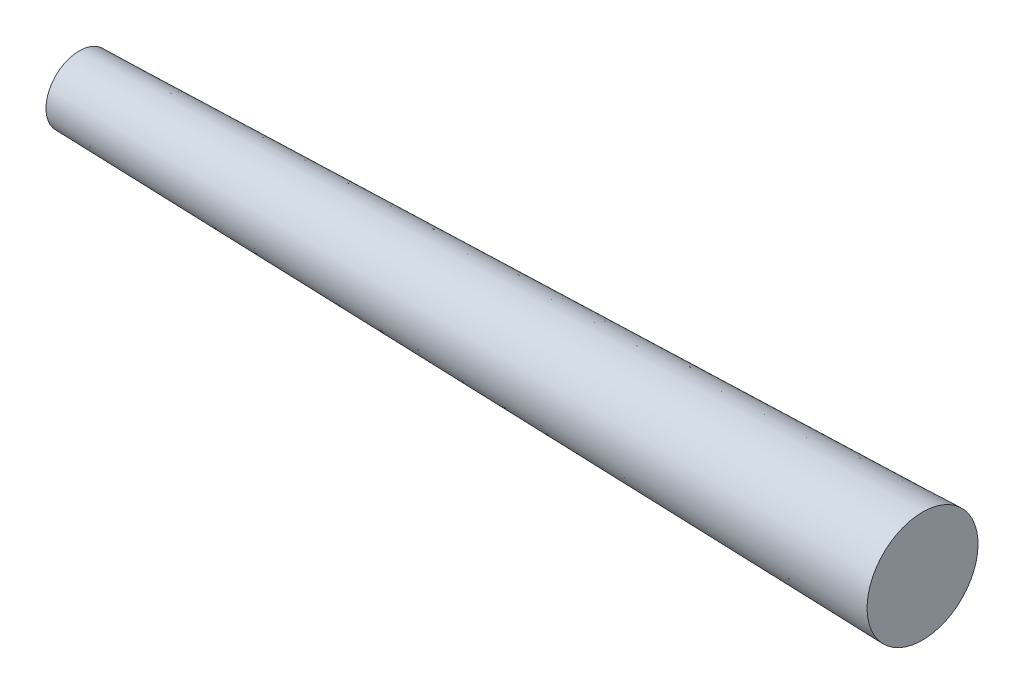
SolidWorks part; units mm, degrees
material "Plain Carbon Steel"
ref_plane "Front Plane" through (0, 0, 0) normal (0, 0, 1) x (1, 0, 0)
ref_plane "Top Plane" through (0, 0, 0) normal (0, 1, 0) x (1, 0, 0)
ref_plane "Right Plane" through (0, 0, 0) normal (1, 0, 0) x (0, 0, -1)
sketch "Taper Pin Profile" plane through (0, 0, 0) normal (0, 0, 1) x (1, 0, 0)
  line L0 (0, 0) -> (-38, 0)
  line L1 (-38, 0) -> (-38, 1.5)
  line L2 (-38, 1.5) -> (0, 2.5)
  line L3 (0, 2.5) -> (0, 0)
  dimension "D1" = 2.5
  dimension "D2" = 1.5
  dimension "D3" = 38
revolve "Taper Pin Ø5-Ø3 x 38" add sketch "Taper Pin Profile" angle 360 about L0
